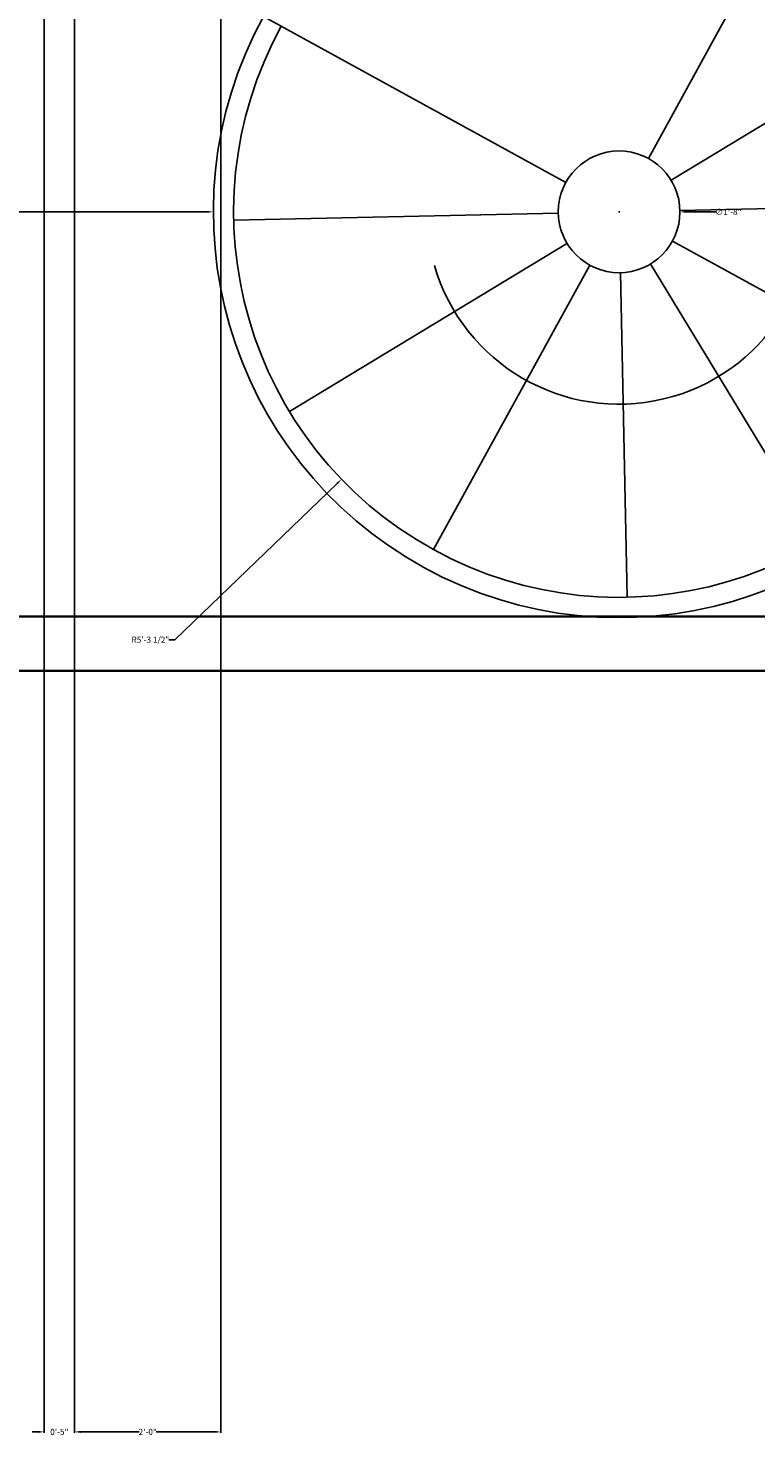
# Model space of a CAD drawing. Units: inches. Extents: x 371 to 1095, y -45 to 1219.
# Tile 3 of 18: x 859 to 979, y -44 to 188. Entities that reach past the tile are written whole.
import ezdxf

# ---------------------------------------------------------------- set-up
doc = ezdxf.new("R2010")
doc.units = ezdxf.units.IN
doc.header["$MEASUREMENT"] = 0
for name, color, linetype, lineweight in [('A-ANNO-DIMS', 2, 'Continuous', 18), ('A-FLOR-STRS', 7, 'Continuous', 25), ('C-SITE-WALL', 40, 'Continuous', 35)]:
    doc.layers.add(name, color=color, linetype=linetype, lineweight=lineweight)
doc.styles.get("Standard").update_dxf_attribs({"font": 'arial.ttf'})
doc.dimstyles.get("Standard").update_dxf_attribs({"dimtxt": 1, "dimasz": 1, "dimexe": 0.18, "dimexo": 0.0625, "dimgap": 0.09, "dimtad": 0, "dimtih": 1, "dimtoh": 1, "dimdec": 0, "dimzin": 0, "dimdsep": 46, "dimlunit": 3, "dimtxsty": 'Standard', "dimcen": 0.09, "dimadec": 0, "dimazin": 0, "dimtfac": 1, "dimtdec": 0, "dimtofl": 0, "dimtmove": 0, "dimatfit": 3, "dimfxl": 1, "dimtolj": 1, "dimtzin": 0, "dimarcsym": 0})

# ---------------------------------------------------------------- blocks, each defined once
blk = doc.blocks.new('Staircase - Spiral')
for p, q in [((0, 4.5), (0, 30)), ((-2.2579, 3.91), (-14.25, 24.681)), ((-3.8566, 2.226), (-24.6818, 14.25)), ((-4.5, 0), (-28.5, 0)), ((4.5, 0), (30, 0)), ((-3.8954, -2.2492), (-24.6818, -14.2502)), ((3.8999, -2.2518), (24.6817, -14.2502)), ((-2.2755, -3.9415), (-14.25, -24.6819)), ((2.2614, -3.9171), (14.25, -24.6819)), ((0, -4.5002), (0, -28.5002)), ((8.5, -10.5002), (11, -9.0002)), ((11, -9.0002), (9.5, -11.5002)), ((9, -11.0002), (8.5, -10.5002)), ((9, -11.0002), (9.5, -11.5002))]:
    blk.add_line(p, q)
blk.add_circle((0, 0), 4.5)
for radius, start, end in [(30, 90, 0), (28.5, 90, 0), (14.2215, 135, 309.2894)]:
    blk.add_arc((0, 0), radius, start, end)
blk = doc.blocks.new('*D60')
at = {"layer": 'A-ANNO-DIMS', "color": 0, "lineweight": -2, "transparency": 16777216}
for p, q in [((866.81, 441.96), (866.81, -43.83)), ((891.01, 441.96), (891.01, -43.83)), ((867.81, -43.65), (877.48, -43.65)), ((890.01, -43.65), (880.33, -43.65))]:
    blk.add_line(p, q, dxfattribs=at)
at = {"layer": 'A-ANNO-DIMS', "color": 0, "transparency": 16777216}
for points in [[(867.81, -43.48), (867.81, -43.82), (866.81, -43.65)], [(890.01, -43.48), (890.01, -43.82), (891.01, -43.65)]]:
    blk.add_solid(points, dxfattribs=at)
at = {"layer": 'Defpoints', "color": 0, "transparency": 16777216}
for p in [(866.81, 442.03), (891.01, 442.03), (891.01, -43.65)]:
    blk.add_point(p, dxfattribs=at)
at = {"layer": 'A-ANNO-DIMS', "color": 0, "transparency": 16777216, "insert": (878.91, -43.65), "char_height": 1, "attachment_point": 5}
blk.add_mtext('\\A1;2\'-0"', dxfattribs=at)
blk = doc.blocks.new('*D61')
at = {"layer": 'A-ANNO-DIMS', "color": 0, "lineweight": -2, "transparency": 16777216}
for p, q in [((861.81, 450.96), (861.81, -43.83)), ((866.81, 450.96), (866.81, -43.83)), ((860.81, -43.65), (859.81, -43.65)), ((867.81, -43.65), (868.81, -43.65))]:
    blk.add_line(p, q, dxfattribs=at)
at = {"layer": 'A-ANNO-DIMS', "color": 0, "transparency": 16777216}
for points in [[(860.81, -43.48), (860.81, -43.82), (861.81, -43.65)], [(867.81, -43.48), (867.81, -43.82), (866.81, -43.65)]]:
    blk.add_solid(points, dxfattribs=at)
at = {"layer": 'Defpoints', "color": 0, "transparency": 16777216}
for p in [(861.81, 451.03), (866.81, 451.03), (866.81, -43.65)]:
    blk.add_point(p, dxfattribs=at)
at = {"layer": 'A-ANNO-DIMS', "color": 0, "transparency": 16777216, "insert": (864.31, -43.65), "char_height": 1, "attachment_point": 5}
blk.add_mtext('\\A1;0\'-5"', dxfattribs=at)
blk = doc.blocks.new('*D66')
at = {"layer": 'A-ANNO-DIMS', "color": 0, "lineweight": -2, "transparency": 16777216}
for p, q in [((849.55, 157.87), (888.76, 157.87)), ((956.69, 157.87), (956.87, 157.87)), ((956.78, 157.78), (956.78, 157.96))]:
    blk.add_line(p, q, dxfattribs=at)
at = {"layer": 'A-ANNO-DIMS', "color": 0, "transparency": 16777216}
blk.add_solid([(888.76, 158.03), (888.76, 157.7), (889.76, 157.87)], dxfattribs=at)
at = {"layer": 'Defpoints', "color": 0, "transparency": 16777216}
for p in [(889.76, 157.87), (956.78, 157.87)]:
    blk.add_point(p, dxfattribs=at)
at = {"layer": 'A-ANNO-DIMS', "color": 0, "transparency": 16777216, "insert": (847.66, 157.87), "char_height": 1, "attachment_point": 5}
blk.add_mtext('\\A1;R5\'-7"', dxfattribs=at)
blk = doc.blocks.new('*D67')
at = {"layer": 'A-ANNO-DIMS', "color": 0, "lineweight": -2, "transparency": 16777216}
for p, q in [((956.69, 157.87), (956.87, 157.87)), ((956.78, 157.78), (956.78, 157.96)), ((883.41, 87.2), (910.2, 113.01)), ((882.41, 87.2), (883.41, 87.2))]:
    blk.add_line(p, q, dxfattribs=at)
at = {"layer": 'A-ANNO-DIMS', "color": 0, "transparency": 16777216}
blk.add_solid([(910.09, 113.13), (910.32, 112.89), (910.92, 113.7)], dxfattribs=at)
at = {"layer": 'Defpoints', "color": 0, "transparency": 16777216}
for p in [(956.78, 157.87), (910.92, 113.7)]:
    blk.add_point(p, dxfattribs=at)
at = {"layer": 'A-ANNO-DIMS', "color": 0, "transparency": 16777216, "insert": (879.35, 87.2), "char_height": 1, "attachment_point": 5}
blk.add_mtext('\\A1;R5\'-3 1/2"', dxfattribs=at)
blk = doc.blocks.new('*D68')
at = {"layer": 'A-ANNO-DIMS', "color": 0, "lineweight": -2, "transparency": 16777216}
for p, q in [((956.69, 157.87), (956.87, 157.87)), ((956.78, 157.78), (956.78, 157.96)), ((972.86, 157.87), (967.83, 157.87))]:
    blk.add_line(p, q, dxfattribs=at)
at = {"layer": 'A-ANNO-DIMS', "color": 0, "transparency": 16777216}
blk.add_solid([(967.83, 158.03), (967.83, 157.7), (966.83, 157.87)], dxfattribs=at)
at = {"layer": 'Defpoints', "color": 0, "transparency": 16777216}
for p in [(946.73, 157.87), (966.83, 157.87)]:
    blk.add_point(p, dxfattribs=at)
at = {"layer": 'A-ANNO-DIMS', "color": 0, "transparency": 16777216, "insert": (974.82, 157.87), "char_height": 1, "attachment_point": 5}
blk.add_mtext('\\A1;∅1\'-8"', dxfattribs=at)

msp = doc.modelspace()

# ---------------------------------------------------------------- linework, layer by layer
at = {"layer": 'C-SITE-WALL'}
for p, q in [((828.28, 91.03), (1023.81, 91.03)), ((822.81, 82.03), (1032.81, 82.03))]:
    msp.add_line(p, q, dxfattribs=at)

# ---------------------------------------------------------------- block references
at = {"layer": 'A-FLOR-STRS', "xscale": 2.233824712970382, "yscale": 2.233824712970382, "zscale": 2.233824712970382, "rotation": 61.2124779579666}
msp.add_blockref('Staircase - Spiral', (956.78, 157.87), dxfattribs=at)

# ---------------------------------------------------------------- dimensions: what is measured, and where the dimension line sits
at = {"layer": 'A-ANNO-DIMS'}
for base, p1, p2, picture, middle in [((866.81, -43.65), (861.81, 451.03), (866.81, 451.03), '*D61', (864.31, -43.65)), ((891.01, -43.65), (866.81, 442.03), (891.01, 442.03), '*D60', (878.91, -43.65))]:
    dim = msp.add_linear_dim(base=base, p1=p1, p2=p2, dimstyle='Standard', override={"dimdec": 1, "dimlfac": 1, "dimrnd": 0, "dimzin": 1, "dimdsep": 46, "dimlunit": 4, "dimfrac": 2}, dxfattribs=at)
    dim.commit()
    dim.dimension.update_dxf_attribs({"geometry": picture, "text_midpoint": middle})
for mpoint, picture, middle in [((889.76, 157.87), '*D66', (849.55, 157.87)), ((910.92, 113.7), '*D67', (879.35, 87.2))]:
    dim = msp.add_radius_dim(center=(956.78, 157.87), mpoint=mpoint, dimstyle='Standard', override={"dimdec": 1, "dimlfac": 1, "dimrnd": 0, "dimzin": 1, "dimdsep": 46, "dimlunit": 4, "dimfrac": 2}, dxfattribs=at)
    dim.commit()
    dim.dimension.update_dxf_attribs({"geometry": picture, "text_midpoint": middle, "dimtype": 164})
dim = msp.add_diameter_dim_2p(p1=(946.73, 157.87), p2=(966.83, 157.87), dimstyle='Standard', override={"dimdec": 1, "dimlfac": 1, "dimrnd": 0, "dimzin": 1, "dimdsep": 46, "dimlunit": 4, "dimfrac": 2}, dxfattribs=at)
dim.commit()
dim.dimension.update_dxf_attribs({"geometry": '*D68', "text_midpoint": (972.86, 157.87), "dimtype": 163})

doc.saveas('drawing.dxf')
